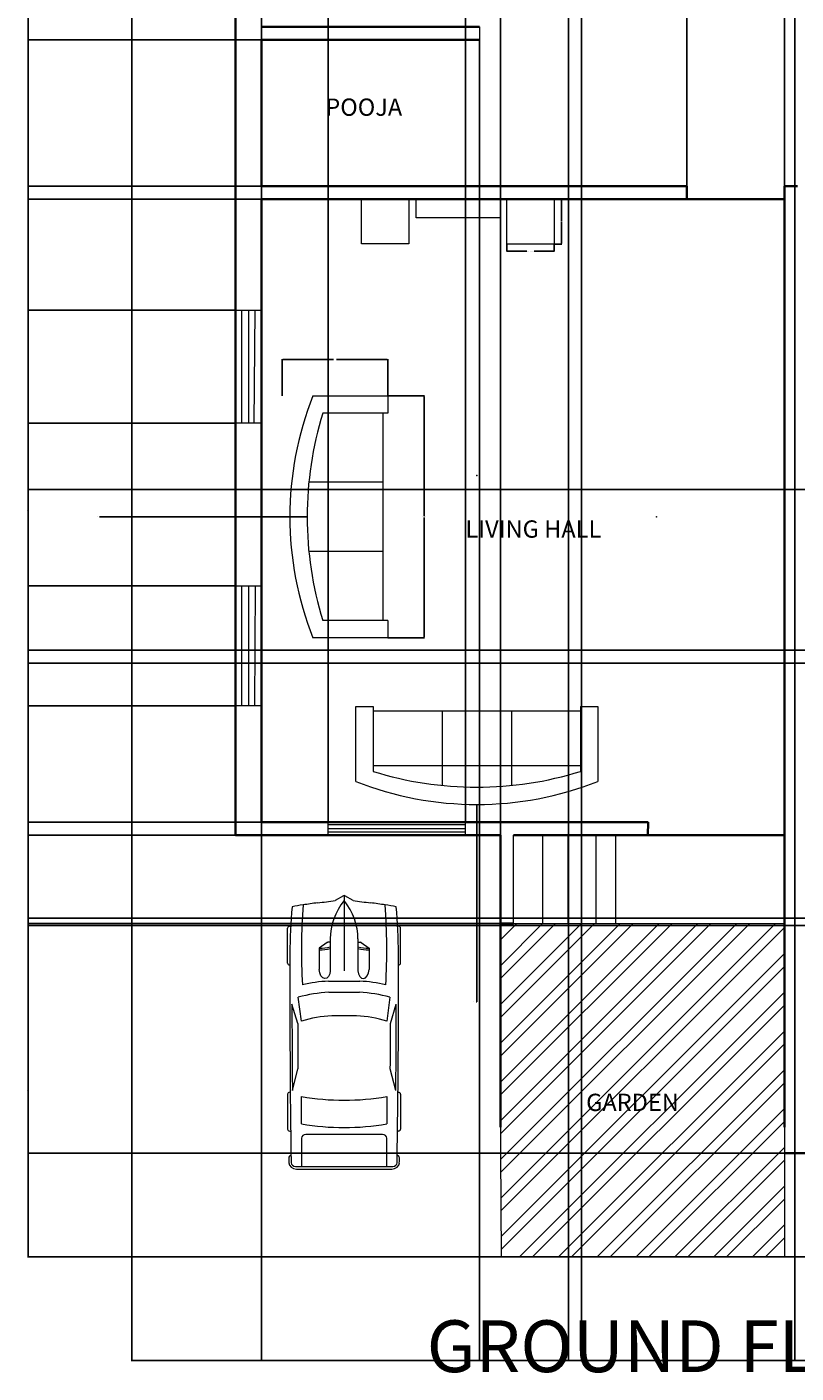
# Model space of a CAD drawing. Units: inches. Extents: x 2621 to 3621, y 1701 to 2465.
# Tile 1 of 6: x 2621 to 2888, y 1701 to 2169. Entities that reach past the tile are written whole.
import ezdxf

# ---------------------------------------------------------------- set-up
doc = ezdxf.new("R2010")
doc.units = ezdxf.units.IN
for name, color, linetype, lineweight in [('A-ANNO-DIMS', 2, 'Continuous', 18), ('A-ANNO-TEXT', 7, 'Continuous', 25), ('A-AREA-IDEN', 7, 'Continuous', 18), ('A-DOOR', 3, 'Continuous', 18), ('A-FLOR-STRS', 30, 'Continuous', 18), ('A-FURN', 8, 'Continuous', 18), ('A-GLAZ', 4, 'Continuous', 18), ('A-WALL', 7, 'Continuous', 35), ('C-PRKG-VEHI', 8, 'Continuous', 13), ('C-PROP', 8, 'Continuous', 25), ('L-PLNT', 94, 'Continuous', 18), ('L-PLNT-PATT', 9, 'Continuous', 13)]:
    doc.layers.add(name, color=color, linetype=linetype, lineweight=lineweight)
doc.styles.get("Standard").update_dxf_attribs({"font": 'arial.ttf'})
doc.dimstyles.get("Standard").update_dxf_attribs({"dimtxt": 0.18, "dimasz": 0.18, "dimexe": 0.18, "dimexo": 0.0625, "dimgap": 0.09, "dimtad": 0, "dimtih": 1, "dimtoh": 1, "dimdec": 4, "dimzin": 0, "dimdsep": 46, "dimtxsty": 'Standard', "dimcen": 0.09, "dimadec": 0, "dimazin": 0, "dimtfac": 1, "dimtdec": 4, "dimtofl": 0, "dimtmove": 0, "dimatfit": 3, "dimfxl": 1, "dimtolj": 1, "dimtzin": 0, "dimarcsym": 0})

# ---------------------------------------------------------------- blocks, each defined once
blk = doc.blocks.new('Sofa - Roundback 7 ft.')
for p, q in [((-12.00002, -32.4421), (-12.00003, -6.5971)), ((11.99997, -32.4421), (11.99998, -6.5971)), ((-36.000027, -34), (-36.000027, -11.4696)), ((-35.999844, -13.3819), (35.9998, -13.3819)), ((35.99998, -34), (35.99998, -11.4696)), ((-36.000027, -32.4421), (35.99998, -32.4421))]:
    blk.add_line(p, q)
for points in [[(-36.000027, -34), (-42.000027, -34), (-42.000027, -8)], [(41.99998, -8), (41.99998, -34), (35.99998, -34)]]:
    blk.add_lwpolyline(points)
for centre, radius, start, end in [((0, -114.25), 114.25, 68.43141, 111.5686), ((-0.00001, -127.1968), 121.1968, 72.72033, 107.2797)]:
    blk.add_arc(centre, radius, start, end)
blk = doc.blocks.new('*U5')
for p, q in [((21.1, 37.41), (21.1, 36.83)), ((46.55, 38.89), (22.35, 38.89)), ((47.8, 37.39), (47.8, 37.41)), ((135.45, 37.07), (135.45, 37.41)), ((136.7, 38.89), (160.9, 38.89)), ((162.15, 37.41), (162.15, 36.77)), ((70.03, 31.54), (86.41, 29.35)), ((87.99, 31.87), (74.76, 35.92)), ((134.31, 35.6), (119.29, 31.78)), ((138.42, 29.35), (157.25, 29.35)), ((186.47, 29.35), (167.01, 29.35)), ((186.47, -33.5), (186.47, 33.5)), ((188.4, -32.76), (188.4, 32.76)), ((164.52, 26.39), (164.52, -26.39)), ((29.77, 9.51), (51.68, 9.51)), ((32.12, 9.51), (32.12, 11.15)), ((32.27, 11.63), (36.13, 17.17)), ((36.13, 17.17), (50.94, 17.17)), ((58.92, -10.77), (58.92, 10.77)), ((66.55, -10.53), (66.55, 10.53)), ((186.47, -10.53), (186.47, 10.53)), ((3.27, 6.13), (0.1, 0.41)), ((82.74, 8.5), (82.74, -8.5)), ((0, 0), (51.68, 0)), ((0.1, -0.41), (3.27, -6.13)), ((29.77, -9.51), (51.68, -9.51)), ((32.12, -9.51), (32.12, -11.15)), ((32.27, -11.63), (36.13, -17.17)), ((36.13, -17.17), (50.94, -17.17)), ((21.1, -37.41), (21.1, -36.83)), ((86.41, -29.35), (70.03, -31.54)), ((87.99, -31.87), (74.76, -35.92)), ((134.31, -35.6), (119.29, -31.78)), ((135.45, -37.07), (135.45, -37.41)), ((157.25, -29.35), (138.42, -29.35)), ((162.15, -37.41), (162.15, -36.77)), ((167.01, -29.35), (186.47, -29.35)), ((46.55, -38.89), (22.35, -38.89)), ((47.8, -37.39), (47.8, -37.41)), ((136.7, -38.89), (160.9, -38.89))]:
    blk.add_line(p, q)
for centre, major_axis, ratio, start_param, end_param in [((41.19, -490.86), (0, 528.23), 0.842304, 0.00281, 0.075598), ((22.35, 37.41), (0, -1.48), 0.842304, 3.141593, 4.712389), ((64.48, -10555.62), (0, 10593.03), 0.842304, -0.013397, 0.002797), ((46.55, 37.41), (0, 1.48), 0.842304, -1.570796, 0), ((136.7, 37.41), (0, -1.48), 0.842304, 3.141593, 4.712389), ((160.9, 37.41), (0, 1.48), 0.842304, -1.570796, 0), ((180.63, 35.84), (0, 2.22), 0.842304, -0.013017, 1.249894), ((64.48, -10556.36), (0, 10595.31), 0.842304, -0.013397, -0.013017), ((183.98, 32.76), (0, -5.25), 0.842304, 1.570796, 3.128196), ((259.18, -27.52), (0, -305.3), 0.842304, 4.528606, 4.561838), ((266.03, -27.52), (0, 313.31), 0.842304, 1.367076, 1.39176), ((37.47, -593.96), (0, -623.33), 0.842304, 3.096046, 3.200911), ((134.4, 5.39), (0, -89.78), 0.842304, 4.449482, 4.652344), ((135.29, 5.39), (0, 81.77), 0.842304, 1.245306, 1.50788), ((64.48, -10555.62), (0, -10591.55), 0.842304, 3.133765, 3.140441), ((149.6, 2.8), (0, -79.58), 0.842304, 4.372215, 4.640744), ((95.79, -3666.35), (0, -3698.24), 0.842304, 3.134049, 3.144098), ((17.08, 0), (0, 147.02), 0.842304, 4.511394, 4.913384), ((35.91, 0), (0, 147.02), 0.842304, 4.511394, 4.913384), ((167.01, 26.39), (0, 2.96), 0.842304, 0, 1.570796), ((183.98, 33.5), (0, -2.96), 0.842304, 1.570796, 3.128196), ((-204.49, 52.4), (0, -250.96), 0.842304, 1.385369, 1.434372), ((29.77, -46.66), (0, 56.17), 0.842304, 0, 0.590319), ((32.75, 11.15), (0, 0.74), 0.842304, 0.879714, 1.570796), ((13.04, 17.01), (0, 27.42), 0.842304, 4.435146, 4.718221), ((14.2, 17.01), (0, 27.42), 0.842304, 4.435146, 4.718221), ((50.79, 13.34), (6.34, -0.36), 0.603834, -1.395552, 1.581315), ((0.62, 0), (0, -0.74), 0.842304, 4.131459, 5.293319), ((-204.49, -52.4), (0, 250.96), 0.842304, -1.434372, -1.385369), ((29.77, 46.66), (0, 56.17), 0.842304, 2.551274, 3.141593), ((149.6, -2.8), (0, -79.58), 0.842304, -1.499151, -1.230623), ((259.18, 27.52), (0, 305.3), 0.842304, 1.721348, 1.754579), ((32.75, -11.15), (0, -0.74), 0.842304, 4.712389, 5.403472), ((13.04, -17.01), (0, -27.42), 0.842304, 1.564964, 1.848039), ((14.2, -17.01), (0, -27.42), 0.842304, 1.564964, 1.848039), ((134.4, -5.39), (0, -89.78), 0.842304, -1.510751, -1.307889), ((135.29, -5.39), (0, -81.77), 0.842304, -1.50788, -1.245306), ((167.01, -26.39), (0, -2.96), 0.842304, 4.712389, 6.283185), ((266.03, 27.52), (0, 313.31), 0.842304, 1.749832, 1.774517), ((37.47, 593.96), (0, -623.33), 0.842304, -0.059319, 0.045547), ((41.19, 490.86), (0, -528.23), 0.842304, -0.075598, -0.00281), ((64.48, 10555.62), (0, 10593.03), 0.842304, 3.138796, 3.15499), ((64.48, 10555.62), (0, -10591.55), 0.842304, 0.001152, 0.007828), ((95.79, 3666.35), (0, -3698.24), 0.842304, -0.002505, 0.007544), ((180.63, -35.84), (0, -2.22), 0.842304, -1.249894, 0.013017), ((183.98, -33.5), (0, 2.96), 0.842304, 3.15499, 4.712389), ((183.98, -32.76), (0, -5.25), 0.842304, 0.013397, 1.570796), ((22.35, -37.41), (0, 1.48), 0.842304, 1.570796, 3.141593), ((46.55, -37.41), (0, -1.48), 0.842304, 0, 1.570796), ((136.7, -37.41), (0, -1.48), 0.842304, -1.570796, 0), ((160.9, -37.41), (0, 1.48), 0.842304, 3.141593, 4.712389), ((64.48, 10556.36), (0, 10595.31), 0.842304, 3.15461, 3.15499)]:
    blk.add_ellipse(centre, major_axis=major_axis, ratio=ratio, start_param=start_param, end_param=end_param)
at = {"extrusion": (0, 0, -1)}
blk.add_ellipse((50.79, -13.34), major_axis=(6.34, 0.36), ratio=0.603834, start_param=-1.395552, end_param=1.581315, dxfattribs=at)
blk = doc.blocks.new('LOT-33X57')
for p, q in [((0, 0), (0, 684)), ((396, 0), (0, 0))]:
    blk.add_line(p, q)
blk = doc.blocks.new('FURN-LIVING-SIDE-UNIT')
blk.add_lwpolyline([(0, 15.51), (16.46, 15.51), (16.46, 0), (0, 0)], close=True)
blk = doc.blocks.new('*D17')
at = {"layer": 'A-ANNO-DIMS', "color": 0, "lineweight": -2, "transparency": 16777216}
for p, q in [((2746.41, 2040.43), (2759.13, 2040.43)), ((2758.95, 2040.25), (2758.95, 1998.61)), ((2758.95, 1956.61), (2758.95, 1998.24)), ((2746.41, 1956.43), (2759.13, 1956.43))]:
    blk.add_line(p, q, dxfattribs=at)
at = {"layer": 'A-ANNO-DIMS', "color": 0, "transparency": 16777216}
for points in [[(2758.92, 2040.25), (2758.98, 2040.25), (2758.95, 2040.43)], [(2758.92, 1956.61), (2758.98, 1956.61), (2758.95, 1956.43)]]:
    blk.add_solid(points, dxfattribs=at)
at = {"layer": 'Defpoints', "color": 0, "transparency": 16777216}
for p in [(2746.35, 2040.43), (2758.95, 2040.43), (2746.35, 1956.43)]:
    blk.add_point(p, dxfattribs=at)
at = {"layer": 'A-ANNO-DIMS', "color": 0, "transparency": 16777216, "insert": (2758.95, 1998.43), "char_height": 0.18, "attachment_point": 5}
blk.add_mtext('\\A1;SOFA 84 TYP.', dxfattribs=at)
blk = doc.blocks.new('*D18')
at = {"layer": 'A-ANNO-DIMS', "color": 0, "lineweight": -2, "transparency": 16777216}
for p, q in [((2709.69, 2040.49), (2709.69, 2053.21)), ((2709.87, 2053.03), (2727.49, 2053.03)), ((2746.17, 2053.03), (2728.55, 2053.03)), ((2746.35, 2040.49), (2746.35, 2053.21))]:
    blk.add_line(p, q, dxfattribs=at)
at = {"layer": 'A-ANNO-DIMS', "color": 0, "transparency": 16777216}
for points in [[(2709.87, 2053.06), (2709.87, 2053), (2709.69, 2053.03)], [(2746.17, 2053.06), (2746.17, 2053), (2746.35, 2053.03)]]:
    blk.add_solid(points, dxfattribs=at)
at = {"layer": 'Defpoints', "color": 0, "transparency": 16777216}
for p in [(2709.69, 2053.03), (2709.69, 2040.43), (2746.35, 2040.43)]:
    blk.add_point(p, dxfattribs=at)
at = {"layer": 'A-ANNO-DIMS', "color": 0, "transparency": 16777216, "insert": (2728.02, 2053.03), "char_height": 0.18, "attachment_point": 5}
blk.add_mtext('\\A1;37 TYP.', dxfattribs=at)
blk = doc.blocks.new('*D31')
at = {"layer": 'A-ANNO-DIMS', "color": 0, "lineweight": -2, "transparency": 16777216}
for p, q in [((2787.64, 2093.1), (2787.64, 2090.52)), ((2787.82, 2090.7), (2794.59, 2090.7)), ((2803.93, 2090.7), (2797.16, 2090.7)), ((2804.11, 2093.1), (2804.11, 2090.52))]:
    blk.add_line(p, q, dxfattribs=at)
at = {"layer": 'A-ANNO-DIMS', "color": 0, "transparency": 16777216}
for points in [[(2787.82, 2090.73), (2787.82, 2090.67), (2787.64, 2090.7)], [(2803.93, 2090.73), (2803.93, 2090.67), (2804.11, 2090.7)]]:
    blk.add_solid(points, dxfattribs=at)
at = {"layer": 'Defpoints', "color": 0, "transparency": 16777216}
for p in [(2787.64, 2093.17), (2804.11, 2093.17), (2804.11, 2090.7)]:
    blk.add_point(p, dxfattribs=at)
at = {"layer": 'A-ANNO-DIMS', "color": 0, "transparency": 16777216, "insert": (2795.87, 2090.7), "char_height": 0.18, "attachment_point": 5}
blk.add_mtext('\\A1;SIDE TABLE 16 TYP.', dxfattribs=at)
blk = doc.blocks.new('*D32')
at = {"layer": 'A-ANNO-DIMS', "color": 0, "lineweight": -2, "transparency": 16777216}
for p, q in [((2804.17, 2108.67), (2806.76, 2108.67)), ((2806.58, 2108.49), (2806.58, 2101.1)), ((2806.58, 2093.35), (2806.58, 2100.74)), ((2804.17, 2093.17), (2806.76, 2093.17))]:
    blk.add_line(p, q, dxfattribs=at)
at = {"layer": 'A-ANNO-DIMS', "color": 0, "transparency": 16777216}
for points in [[(2806.55, 2108.49), (2806.61, 2108.49), (2806.58, 2108.67)], [(2806.55, 2093.35), (2806.61, 2093.35), (2806.58, 2093.17)]]:
    blk.add_solid(points, dxfattribs=at)
at = {"layer": 'Defpoints', "color": 0, "transparency": 16777216}
for p in [(2804.11, 2108.67), (2806.58, 2108.67), (2804.11, 2093.17)]:
    blk.add_point(p, dxfattribs=at)
at = {"layer": 'A-ANNO-DIMS', "color": 0, "transparency": 16777216, "insert": (2806.58, 2100.92), "char_height": 0.18, "attachment_point": 5}
blk.add_mtext('\\A1;16 TYP.', dxfattribs=at)
blk = doc.blocks.new('*D35')
at = {"layer": 'A-ANNO-DIMS', "color": 0, "lineweight": -2, "transparency": 16777216}
for p, q in [((2657.52, 1741.34), (2657.52, 1705.2)), ((3053.52, 1741.34), (3053.52, 1705.2)), ((2657.7, 1705.38), (2855.23, 1705.38)), ((3053.34, 1705.38), (2855.81, 1705.38))]:
    blk.add_line(p, q, dxfattribs=at)
at = {"layer": 'A-ANNO-DIMS', "color": 0, "transparency": 16777216}
for points in [[(2657.7, 1705.41), (2657.7, 1705.35), (2657.52, 1705.38)], [(3053.34, 1705.41), (3053.34, 1705.35), (3053.52, 1705.38)]]:
    blk.add_solid(points, dxfattribs=at)
at = {"layer": 'Defpoints', "color": 0, "transparency": 16777216}
for p in [(2657.52, 1741.4), (3053.52, 1741.4), (3053.52, 1705.38)]:
    blk.add_point(p, dxfattribs=at)
at = {"layer": 'A-ANNO-DIMS', "color": 0, "transparency": 16777216, "insert": (2855.52, 1705.38), "char_height": 0.18, "attachment_point": 5}
blk.add_mtext('\\A1;396', dxfattribs=at)
blk = doc.blocks.new('*D36')
at = {"layer": 'A-ANNO-DIMS', "color": 0, "lineweight": -2, "transparency": 16777216}
for p, q in [((2657.46, 2425.4), (2621.31, 2425.4)), ((2621.49, 2425.22), (2621.49, 2083.58)), ((2621.49, 1741.58), (2621.49, 2083.22)), ((2657.46, 1741.4), (2621.31, 1741.4))]:
    blk.add_line(p, q, dxfattribs=at)
at = {"layer": 'A-ANNO-DIMS', "color": 0, "transparency": 16777216}
for points in [[(2621.46, 2425.22), (2621.52, 2425.22), (2621.49, 2425.4)], [(2621.46, 1741.58), (2621.52, 1741.58), (2621.49, 1741.4)]]:
    blk.add_solid(points, dxfattribs=at)
at = {"layer": 'Defpoints', "color": 0, "transparency": 16777216}
for p in [(2621.49, 2425.4), (2657.52, 2425.4), (2657.52, 1741.4)]:
    blk.add_point(p, dxfattribs=at)
at = {"layer": 'A-ANNO-DIMS', "color": 0, "transparency": 16777216, "insert": (2621.49, 2083.4), "char_height": 0.18, "attachment_point": 5}
blk.add_mtext('\\A1;684', dxfattribs=at)
blk = doc.blocks.new('*D42')
at = {"layer": 'A-ANNO-DIMS', "color": 0, "lineweight": -2, "transparency": 16777216}
for p, q in [((2702.52, 2380.34), (2702.52, 1705.2)), ((2809.02, 2380.34), (2809.02, 1705.2)), ((2702.7, 1705.38), (2755.38, 1705.38)), ((2808.84, 1705.38), (2756.15, 1705.38))]:
    blk.add_line(p, q, dxfattribs=at)
at = {"layer": 'A-ANNO-DIMS', "color": 0, "transparency": 16777216}
for points in [[(2702.7, 1705.41), (2702.7, 1705.35), (2702.52, 1705.38)], [(2808.84, 1705.41), (2808.84, 1705.35), (2809.02, 1705.38)]]:
    blk.add_solid(points, dxfattribs=at)
at = {"layer": 'Defpoints', "color": 0, "transparency": 16777216}
for p in [(2702.52, 2380.4), (2809.02, 2380.4), (2809.02, 1705.38)]:
    blk.add_point(p, dxfattribs=at)
at = {"layer": 'A-ANNO-DIMS', "color": 0, "transparency": 16777216, "insert": (2755.77, 1705.38), "char_height": 0.18, "attachment_point": 5}
blk.add_mtext('\\A1;106.5', dxfattribs=at)
blk = doc.blocks.new('*D43')
at = {"layer": 'A-ANNO-DIMS', "color": 0, "lineweight": -2, "transparency": 16777216}
for p, q in [((2813.52, 2380.34), (2813.52, 1705.2)), ((2887.57, 2380.34), (2887.57, 1705.2)), ((2813.7, 1705.38), (2850.15, 1705.38)), ((2887.39, 1705.38), (2850.94, 1705.38))]:
    blk.add_line(p, q, dxfattribs=at)
at = {"layer": 'A-ANNO-DIMS', "color": 0, "transparency": 16777216}
for points in [[(2813.7, 1705.41), (2813.7, 1705.35), (2813.52, 1705.38)], [(2887.39, 1705.41), (2887.39, 1705.35), (2887.57, 1705.38)]]:
    blk.add_solid(points, dxfattribs=at)
at = {"layer": 'Defpoints', "color": 0, "transparency": 16777216}
for p in [(2813.52, 2380.4), (2887.57, 2380.4), (2887.57, 1705.38)]:
    blk.add_point(p, dxfattribs=at)
at = {"layer": 'A-ANNO-DIMS', "color": 0, "transparency": 16777216, "insert": (2850.55, 1705.38), "char_height": 0.18, "attachment_point": 5}
blk.add_mtext('\\A1;74.05', dxfattribs=at)
blk = doc.blocks.new('*D49')
at = {"layer": 'A-ANNO-DIMS', "color": 0, "lineweight": -2, "transparency": 16777216}
for p, q in [((2702.52, 2164.01), (2702.52, 1705.2)), ((2778.15, 2164.01), (2778.15, 1705.2)), ((2702.7, 1705.38), (2739.94, 1705.38)), ((2777.97, 1705.38), (2740.73, 1705.38))]:
    blk.add_line(p, q, dxfattribs=at)
at = {"layer": 'A-ANNO-DIMS', "color": 0, "transparency": 16777216}
for points in [[(2702.7, 1705.41), (2702.7, 1705.35), (2702.52, 1705.38)], [(2777.97, 1705.41), (2777.97, 1705.35), (2778.15, 1705.38)]]:
    blk.add_solid(points, dxfattribs=at)
at = {"layer": 'Defpoints', "color": 0, "transparency": 16777216}
for p in [(2702.52, 2164.07), (2778.15, 2164.07), (2778.15, 1705.38)]:
    blk.add_point(p, dxfattribs=at)
at = {"layer": 'A-ANNO-DIMS', "color": 0, "transparency": 16777216, "insert": (2740.33, 1705.38), "char_height": 0.18, "attachment_point": 5}
blk.add_mtext('\\A1;75.63', dxfattribs=at)
blk = doc.blocks.new('*D50')
at = {"layer": 'A-ANNO-DIMS', "color": 0, "lineweight": -2, "transparency": 16777216}
for p, q in [((2702.46, 2164.07), (2621.31, 2164.07)), ((2621.49, 2163.89), (2621.49, 2138.84)), ((2621.49, 2113.43), (2621.49, 2138.48)), ((2702.46, 2113.25), (2621.31, 2113.25))]:
    blk.add_line(p, q, dxfattribs=at)
at = {"layer": 'A-ANNO-DIMS', "color": 0, "transparency": 16777216}
for points in [[(2621.46, 2163.89), (2621.52, 2163.89), (2621.49, 2164.07)], [(2621.46, 2113.43), (2621.52, 2113.43), (2621.49, 2113.25)]]:
    blk.add_solid(points, dxfattribs=at)
at = {"layer": 'Defpoints', "color": 0, "transparency": 16777216}
for p in [(2621.49, 2164.07), (2702.52, 2164.07), (2702.52, 2113.25)]:
    blk.add_point(p, dxfattribs=at)
at = {"layer": 'A-ANNO-DIMS', "color": 0, "transparency": 16777216, "insert": (2621.49, 2138.66), "char_height": 0.18, "attachment_point": 5}
blk.add_mtext('\\A1;50.82', dxfattribs=at)
blk = doc.blocks.new('*D51')
at = {"layer": 'A-ANNO-DIMS', "color": 0, "lineweight": -2, "transparency": 16777216}
for p, q in [((2702.46, 2108.75), (2621.31, 2108.75)), ((2621.49, 2108.57), (2621.49, 2000.76)), ((2621.49, 1892.58), (2621.49, 2000.39)), ((2702.46, 1892.4), (2621.31, 1892.4))]:
    blk.add_line(p, q, dxfattribs=at)
at = {"layer": 'A-ANNO-DIMS', "color": 0, "transparency": 16777216}
for points in [[(2621.46, 2108.57), (2621.52, 2108.57), (2621.49, 2108.75)], [(2621.46, 1892.58), (2621.52, 1892.58), (2621.49, 1892.4)]]:
    blk.add_solid(points, dxfattribs=at)
at = {"layer": 'Defpoints', "color": 0, "transparency": 16777216}
for p in [(2621.49, 2108.75), (2702.52, 2108.75), (2702.52, 1892.4)]:
    blk.add_point(p, dxfattribs=at)
at = {"layer": 'A-ANNO-DIMS', "color": 0, "transparency": 16777216, "insert": (2621.49, 2000.58), "char_height": 0.18, "attachment_point": 5}
blk.add_mtext('\\A1;216.35', dxfattribs=at)
blk = doc.blocks.new('*D52')
at = {"layer": 'A-ANNO-DIMS', "color": 0, "lineweight": -2, "transparency": 16777216}
for p, q in [((2702.52, 1892.46), (2702.52, 2461.61)), ((2702.7, 2461.43), (2792.8, 2461.43)), ((2883.82, 2461.43), (2793.71, 2461.43)), ((2884, 1887.96), (2884, 2461.61))]:
    blk.add_line(p, q, dxfattribs=at)
at = {"layer": 'A-ANNO-DIMS', "color": 0, "transparency": 16777216}
for points in [[(2702.7, 2461.46), (2702.7, 2461.4), (2702.52, 2461.43)], [(2883.82, 2461.46), (2883.82, 2461.4), (2884, 2461.43)]]:
    blk.add_solid(points, dxfattribs=at)
at = {"layer": 'Defpoints', "color": 0, "transparency": 16777216}
for p in [(2884, 2461.43), (2702.52, 1892.4), (2884, 1887.9)]:
    blk.add_point(p, dxfattribs=at)
at = {"layer": 'A-ANNO-DIMS', "color": 0, "transparency": 16777216, "insert": (2793.26, 2461.43), "char_height": 0.18, "attachment_point": 5}
blk.add_mtext('\\A1;181.48', dxfattribs=at)
blk = doc.blocks.new('*D54')
at = {"layer": 'A-ANNO-DIMS', "color": 0, "lineweight": -2, "transparency": 16777216}
for p, q in [((3008.46, 1856.54), (2621.31, 1856.54)), ((2621.49, 1856.36), (2621.49, 1817.15)), ((2621.49, 1777.58), (2621.49, 1816.79)), ((3008.46, 1777.4), (2621.31, 1777.4))]:
    blk.add_line(p, q, dxfattribs=at)
at = {"layer": 'A-ANNO-DIMS', "color": 0, "transparency": 16777216}
for points in [[(2621.46, 1856.36), (2621.52, 1856.36), (2621.49, 1856.54)], [(2621.46, 1777.58), (2621.52, 1777.58), (2621.49, 1777.4)]]:
    blk.add_solid(points, dxfattribs=at)
at = {"layer": 'Defpoints', "color": 0, "transparency": 16777216}
for p in [(2621.49, 1856.54), (3008.52, 1856.54), (3008.52, 1777.4)]:
    blk.add_point(p, dxfattribs=at)
at = {"layer": 'A-ANNO-DIMS', "color": 0, "transparency": 16777216, "insert": (2621.49, 1816.97), "char_height": 0.18, "attachment_point": 5}
blk.add_mtext('\\A1;79.14', dxfattribs=at)
blk = doc.blocks.new('*D55')
at = {"layer": 'A-ANNO-DIMS', "color": 0, "lineweight": -2, "transparency": 16777216}
for p, q in [((3008.46, 1947.58), (2621.31, 1947.58)), ((2621.49, 1947.4), (2621.49, 1903.51)), ((2621.49, 1859.26), (2621.49, 1903.15)), ((3008.46, 1859.08), (2621.31, 1859.08))]:
    blk.add_line(p, q, dxfattribs=at)
at = {"layer": 'A-ANNO-DIMS', "color": 0, "transparency": 16777216}
for points in [[(2621.46, 1947.4), (2621.52, 1947.4), (2621.49, 1947.58)], [(2621.46, 1859.26), (2621.52, 1859.26), (2621.49, 1859.08)]]:
    blk.add_solid(points, dxfattribs=at)
at = {"layer": 'Defpoints', "color": 0, "transparency": 16777216}
for p in [(2621.49, 1947.58), (3008.52, 1947.58), (3008.52, 1859.08)]:
    blk.add_point(p, dxfattribs=at)
at = {"layer": 'A-ANNO-DIMS', "color": 0, "transparency": 16777216, "insert": (2621.49, 1903.33), "char_height": 0.18, "attachment_point": 5}
blk.add_mtext('\\A1;88.5', dxfattribs=at)
blk = doc.blocks.new('*D58')
at = {"layer": 'A-ANNO-DIMS', "color": 0, "lineweight": -2, "transparency": 16777216}
for p, q in [((2933.41, 2007.9), (2621.31, 2007.9)), ((2621.49, 2007.72), (2621.49, 1980.17)), ((2621.49, 1952.26), (2621.49, 1979.81)), ((2933.41, 1952.08), (2621.31, 1952.08))]:
    blk.add_line(p, q, dxfattribs=at)
at = {"layer": 'A-ANNO-DIMS', "color": 0, "transparency": 16777216}
for points in [[(2621.46, 2007.72), (2621.52, 2007.72), (2621.49, 2007.9)], [(2621.46, 1952.26), (2621.52, 1952.26), (2621.49, 1952.08)]]:
    blk.add_solid(points, dxfattribs=at)
at = {"layer": 'Defpoints', "color": 0, "transparency": 16777216}
for p in [(2621.49, 2007.9), (2933.47, 2007.9), (2933.47, 1952.08)]:
    blk.add_point(p, dxfattribs=at)
at = {"layer": 'A-ANNO-DIMS', "color": 0, "transparency": 16777216, "insert": (2621.49, 1979.99), "char_height": 0.18, "attachment_point": 5}
blk.add_mtext('\\A1;55.82', dxfattribs=at)
blk = doc.blocks.new('*D61')
at = {"layer": 'A-ANNO-DIMS', "color": 0, "lineweight": -2, "transparency": 16777216}
for p, q in [((2785.46, 1857.23), (2785.46, 2461.61)), ((2785.64, 2461.43), (2834.33, 2461.43)), ((2883.82, 2461.43), (2835.12, 2461.43)), ((2884, 1857.23), (2884, 2461.61))]:
    blk.add_line(p, q, dxfattribs=at)
at = {"layer": 'A-ANNO-DIMS', "color": 0, "transparency": 16777216}
for points in [[(2785.64, 2461.46), (2785.64, 2461.4), (2785.46, 2461.43)], [(2883.82, 2461.46), (2883.82, 2461.4), (2884, 2461.43)]]:
    blk.add_solid(points, dxfattribs=at)
at = {"layer": 'Defpoints', "color": 0, "transparency": 16777216}
for p in [(2884, 2461.43), (2785.46, 1857.17), (2884, 1857.17)]:
    blk.add_point(p, dxfattribs=at)
at = {"layer": 'A-ANNO-DIMS', "color": 0, "transparency": 16777216, "insert": (2834.73, 2461.43), "char_height": 0.18, "attachment_point": 5}
blk.add_mtext('\\A1;98.54', dxfattribs=at)
blk = doc.blocks.new('*D62')
at = {"layer": 'A-ANNO-DIMS', "color": 0, "lineweight": -2, "transparency": 16777216}
for p, q in [((2785.4, 1857.17), (2621.31, 1857.17)), ((2621.49, 1856.99), (2621.49, 1799.47)), ((2621.49, 1741.58), (2621.49, 1799.1)), ((2785.66, 1741.4), (2621.31, 1741.4))]:
    blk.add_line(p, q, dxfattribs=at)
at = {"layer": 'A-ANNO-DIMS', "color": 0, "transparency": 16777216}
for points in [[(2621.46, 1856.99), (2621.52, 1856.99), (2621.49, 1857.17)], [(2621.46, 1741.58), (2621.52, 1741.58), (2621.49, 1741.4)]]:
    blk.add_solid(points, dxfattribs=at)
at = {"layer": 'Defpoints', "color": 0, "transparency": 16777216}
for p in [(2621.49, 1857.17), (2785.46, 1857.17), (2785.72, 1741.4)]:
    blk.add_point(p, dxfattribs=at)
at = {"layer": 'A-ANNO-DIMS', "color": 0, "transparency": 16777216, "insert": (2621.49, 1799.28), "char_height": 0.18, "attachment_point": 5}
blk.add_mtext('\\A1;115.77', dxfattribs=at)
blk = doc.blocks.new('*D87')
at = {"layer": 'A-ANNO-DIMS', "color": 0, "lineweight": -2, "transparency": 16777216}
for p, q in [((2693.46, 1932.75), (2621.31, 1932.75)), ((2621.49, 1932.57), (2621.49, 1910.51)), ((2621.49, 1888.08), (2621.49, 1910.14)), ((2693.46, 1887.9), (2621.31, 1887.9))]:
    blk.add_line(p, q, dxfattribs=at)
at = {"layer": 'A-ANNO-DIMS', "color": 0, "transparency": 16777216}
for points in [[(2621.46, 1932.57), (2621.52, 1932.57), (2621.49, 1932.75)], [(2621.46, 1888.08), (2621.52, 1888.08), (2621.49, 1887.9)]]:
    blk.add_solid(points, dxfattribs=at)
at = {"layer": 'Defpoints', "color": 0, "transparency": 16777216}
for p in [(2621.49, 1932.75), (2693.52, 1932.75), (2693.52, 1887.9)]:
    blk.add_point(p, dxfattribs=at)
at = {"layer": 'A-ANNO-DIMS', "color": 0, "transparency": 16777216, "insert": (2621.49, 1910.32), "char_height": 0.18, "attachment_point": 5}
blk.add_mtext('\\A1;44.85', dxfattribs=at)
blk = doc.blocks.new('*D88')
at = {"layer": 'A-ANNO-DIMS', "color": 0, "lineweight": -2, "transparency": 16777216}
for p, q in [((2693.46, 1974.42), (2621.31, 1974.42)), ((2621.49, 1974.24), (2621.49, 1953.77)), ((2621.49, 1932.93), (2621.49, 1953.4)), ((2693.46, 1932.75), (2621.31, 1932.75))]:
    blk.add_line(p, q, dxfattribs=at)
at = {"layer": 'A-ANNO-DIMS', "color": 0, "transparency": 16777216}
for points in [[(2621.46, 1974.24), (2621.52, 1974.24), (2621.49, 1974.42)], [(2621.46, 1932.93), (2621.52, 1932.93), (2621.49, 1932.75)]]:
    blk.add_solid(points, dxfattribs=at)
at = {"layer": 'Defpoints', "color": 0, "transparency": 16777216}
for p in [(2621.49, 1974.42), (2693.52, 1974.42), (2693.52, 1932.75)]:
    blk.add_point(p, dxfattribs=at)
at = {"layer": 'A-ANNO-DIMS', "color": 0, "transparency": 16777216, "insert": (2621.49, 1953.59), "char_height": 0.18, "attachment_point": 5}
blk.add_mtext('\\A1;41.67', dxfattribs=at)
blk = doc.blocks.new('*D89')
at = {"layer": 'A-ANNO-DIMS', "color": 0, "lineweight": -2, "transparency": 16777216}
for p, q in [((2693.46, 2030.98), (2621.31, 2030.98)), ((2621.49, 2030.8), (2621.49, 2002.88)), ((2621.49, 1974.6), (2621.49, 2002.52)), ((2693.46, 1974.42), (2621.31, 1974.42))]:
    blk.add_line(p, q, dxfattribs=at)
at = {"layer": 'A-ANNO-DIMS', "color": 0, "transparency": 16777216}
for points in [[(2621.46, 2030.8), (2621.52, 2030.8), (2621.49, 2030.98)], [(2621.46, 1974.6), (2621.52, 1974.6), (2621.49, 1974.42)]]:
    blk.add_solid(points, dxfattribs=at)
at = {"layer": 'Defpoints', "color": 0, "transparency": 16777216}
for p in [(2621.49, 2030.98), (2693.52, 2030.98), (2693.52, 1974.42)]:
    blk.add_point(p, dxfattribs=at)
at = {"layer": 'A-ANNO-DIMS', "color": 0, "transparency": 16777216, "insert": (2621.49, 2002.7), "char_height": 0.18, "attachment_point": 5}
blk.add_mtext('\\A1;56.55', dxfattribs=at)
blk = doc.blocks.new('*D90')
at = {"layer": 'A-ANNO-DIMS', "color": 0, "lineweight": -2, "transparency": 16777216}
for p, q in [((2693.46, 2070.17), (2621.31, 2070.17)), ((2621.49, 2069.99), (2621.49, 2050.75)), ((2621.49, 2031.16), (2621.49, 2050.39)), ((2693.46, 2030.98), (2621.31, 2030.98))]:
    blk.add_line(p, q, dxfattribs=at)
at = {"layer": 'A-ANNO-DIMS', "color": 0, "transparency": 16777216}
for points in [[(2621.46, 2069.99), (2621.52, 2069.99), (2621.49, 2070.17)], [(2621.46, 2031.16), (2621.52, 2031.16), (2621.49, 2030.98)]]:
    blk.add_solid(points, dxfattribs=at)
at = {"layer": 'Defpoints', "color": 0, "transparency": 16777216}
for p in [(2621.49, 2070.17), (2693.52, 2070.17), (2693.52, 2030.98)]:
    blk.add_point(p, dxfattribs=at)
at = {"layer": 'A-ANNO-DIMS', "color": 0, "transparency": 16777216, "insert": (2621.49, 2050.57), "char_height": 0.18, "attachment_point": 5}
blk.add_mtext('\\A1;39.19', dxfattribs=at)
blk = doc.blocks.new('*D98')
at = {"layer": 'A-ANNO-DIMS', "color": 0, "lineweight": -2, "transparency": 16777216}
for p, q in [((2702.52, 1892.46), (2702.52, 2461.61)), ((2702.7, 2461.43), (2713.72, 2461.43)), ((2725.53, 2461.43), (2714.51, 2461.43)), ((2725.71, 1892.46), (2725.71, 2461.61))]:
    blk.add_line(p, q, dxfattribs=at)
at = {"layer": 'A-ANNO-DIMS', "color": 0, "transparency": 16777216}
for points in [[(2702.7, 2461.46), (2702.7, 2461.4), (2702.52, 2461.43)], [(2725.53, 2461.46), (2725.53, 2461.4), (2725.71, 2461.43)]]:
    blk.add_solid(points, dxfattribs=at)
at = {"layer": 'Defpoints', "color": 0, "transparency": 16777216}
for p in [(2725.71, 2461.43), (2702.52, 1892.4), (2725.71, 1892.4)]:
    blk.add_point(p, dxfattribs=at)
at = {"layer": 'A-ANNO-DIMS', "color": 0, "transparency": 16777216, "insert": (2714.11, 2461.43), "char_height": 0.18, "attachment_point": 5}
blk.add_mtext('\\A1;23.19', dxfattribs=at)
blk = doc.blocks.new('*D99')
at = {"layer": 'A-ANNO-DIMS', "color": 0, "lineweight": -2, "transparency": 16777216}
for p, q in [((2725.71, 1892.46), (2725.71, 2461.61)), ((2725.89, 2461.43), (2749.13, 2461.43)), ((2773.18, 2461.43), (2749.93, 2461.43)), ((2773.36, 1892.46), (2773.36, 2461.61))]:
    blk.add_line(p, q, dxfattribs=at)
at = {"layer": 'A-ANNO-DIMS', "color": 0, "transparency": 16777216}
for points in [[(2725.89, 2461.46), (2725.89, 2461.4), (2725.71, 2461.43)], [(2773.18, 2461.46), (2773.18, 2461.4), (2773.36, 2461.43)]]:
    blk.add_solid(points, dxfattribs=at)
at = {"layer": 'Defpoints', "color": 0, "transparency": 16777216}
for p in [(2773.36, 2461.43), (2725.71, 1892.4), (2773.36, 1892.4)]:
    blk.add_point(p, dxfattribs=at)
at = {"layer": 'A-ANNO-DIMS', "color": 0, "transparency": 16777216, "insert": (2749.53, 2461.43), "char_height": 0.18, "attachment_point": 5}
blk.add_mtext('\\A1;47.65', dxfattribs=at)
blk = doc.blocks.new('*D100')
at = {"layer": 'A-ANNO-DIMS', "color": 0, "lineweight": -2, "transparency": 16777216}
for p, q in [((2850.13, 2113.32), (2850.13, 2461.61)), ((2850.31, 2461.43), (2866.67, 2461.43)), ((2883.82, 2461.43), (2867.45, 2461.43)), ((2884, 2113.32), (2884, 2461.61))]:
    blk.add_line(p, q, dxfattribs=at)
at = {"layer": 'A-ANNO-DIMS', "color": 0, "transparency": 16777216}
for points in [[(2850.31, 2461.46), (2850.31, 2461.4), (2850.13, 2461.43)], [(2883.82, 2461.46), (2883.82, 2461.4), (2884, 2461.43)]]:
    blk.add_solid(points, dxfattribs=at)
at = {"layer": 'Defpoints', "color": 0, "transparency": 16777216}
for p in [(2884, 2461.43), (2850.13, 2113.25), (2884, 2113.25)]:
    blk.add_point(p, dxfattribs=at)
at = {"layer": 'A-ANNO-DIMS', "color": 0, "transparency": 16777216, "insert": (2867.06, 2461.43), "char_height": 0.18, "attachment_point": 5}
blk.add_mtext('\\A1;33.87', dxfattribs=at)
blk = doc.blocks.new('*D106')
at = {"layer": 'A-ANNO-DIMS', "color": 0, "lineweight": -2, "transparency": 16777216}
for p, q in [((2646.31, 1998.43), (2718.17, 1998.43)), ((2839.46, 1998.43), (2839.64, 1998.43)), ((2839.55, 1998.34), (2839.55, 1998.52))]:
    blk.add_line(p, q, dxfattribs=at)
at = {"layer": 'A-ANNO-DIMS', "color": 0, "transparency": 16777216}
blk.add_solid([(2718.17, 1998.46), (2718.17, 1998.4), (2718.35, 1998.43)], dxfattribs=at)
at = {"layer": 'Defpoints', "color": 0, "transparency": 16777216}
for p in [(2718.35, 1998.43), (2839.55, 1998.43)]:
    blk.add_point(p, dxfattribs=at)
at = {"layer": 'A-ANNO-DIMS', "color": 0, "transparency": 16777216, "insert": (2645.63, 1998.43), "char_height": 0.18, "attachment_point": 5}
blk.add_mtext('\\A1;2X R121.2', dxfattribs=at)
blk = doc.blocks.new('*D107')
at = {"layer": 'A-ANNO-DIMS', "color": 0, "lineweight": -2, "transparency": 16777216}
for p, q in [((2777.14, 2012.78), (2777.32, 2012.78)), ((2777.23, 2012.69), (2777.23, 2012.87)), ((2777.23, 1829.98), (2777.23, 1898.35)), ((2777.05, 1829.98), (2777.23, 1829.98))]:
    blk.add_line(p, q, dxfattribs=at)
at = {"layer": 'A-ANNO-DIMS', "color": 0, "transparency": 16777216}
blk.add_solid([(2777.2, 1898.35), (2777.26, 1898.35), (2777.23, 1898.53)], dxfattribs=at)
at = {"layer": 'Defpoints', "color": 0, "transparency": 16777216}
for p in [(2777.23, 2012.78), (2777.23, 1898.53)]:
    blk.add_point(p, dxfattribs=at)
at = {"layer": 'A-ANNO-DIMS', "color": 0, "transparency": 16777216, "insert": (2776.3, 1829.98), "char_height": 0.18, "attachment_point": 5}
blk.add_mtext('\\A1;2X R114.25', dxfattribs=at)

msp = doc.modelspace()

# ---------------------------------------------------------------- hatches: boundary and pattern name
at = {"layer": 'L-PLNT-PATT'}
h = msp.add_hatch(dxfattribs=at)
h.set_pattern_fill('ANSI32', color=256)
h.paths.add_polyline_path([(2883.995, 1857.1678), (2789.9592, 1857.1678), (2785.4592, 1857.1678), (2785.4592, 1786.4015), (2785.4592, 1777.4015), (2785.7201, 1741.4015), (2883.995, 1741.4015), (2883.995, 1786.4015)])

# ---------------------------------------------------------------- linework, layer by layer
at = {"layer": 'A-DOOR'}
msp.add_line((2778.1477, 2168.5709), (2778.1477, 2113.2527), dxfattribs=at)
at = {"layer": 'A-FLOR-STRS'}
for p, q in [((2789.9592, 1857.1678), (2789.9592, 1887.8987)), ((2800.1093, 1857.1678), (2800.1093, 1887.8987)), ((2808.9654, 1857.1678), (2808.9654, 1887.8987)), ((2818.6518, 1857.1678), (2818.6518, 1887.8987)), ((2825.466, 1857.1678), (2825.466, 1887.8987)), ((2789.9592, 1857.1678), (2883.995, 1857.1678))]:
    msp.add_line(p, q, dxfattribs=at)
at = {"layer": 'A-FURN'}
msp.add_lwpolyline([(2756.1697, 2108.7527), (2785.4943, 2108.7527), (2785.4943, 2102.2982), (2756.1697, 2102.2982)], close=True, dxfattribs=at)
at = {"layer": 'A-GLAZ'}
for p, q in [((2695.6642, 2030.9765), (2695.6642, 2070.168)), ((2698.0184, 2070.168), (2698.0184, 2030.9765)), ((2700.1954, 2070.168), (2699.828, 2030.9765)), ((2695.662, 1932.7498), (2695.7383, 1974.4218)), ((2698.0184, 1974.4218), (2698.0184, 1932.7498)), ((2700.2073, 1932.7498), (2700.3939, 1974.4218)), ((2725.7097, 1887.8987), (2725.7097, 1892.3987)), ((2773.3373, 1891.4514), (2725.7097, 1891.4514)), ((2725.7097, 1890.1487), (2773.312, 1890.1487)), ((2725.7097, 1889.0239), (2773.2901, 1889.0239)), ((2773.2683, 1887.8987), (2773.3557, 1892.3987))]:
    msp.add_line(p, q, dxfattribs=at)
for points in [[(2693.5184, 2070.168), (2702.5184, 2070.168), (2702.5184, 2030.9765), (2693.5184, 2030.9765)], [(2693.5184, 1974.4218), (2702.5184, 1974.4218), (2702.5184, 1932.7498), (2693.5184, 1932.7498)]]:
    msp.add_lwpolyline(points, close=True, dxfattribs=at)
at = {"layer": 'A-WALL'}
for p, q in [((2693.5184, 2425.4015), (2693.5184, 1887.8987)), ((2702.5184, 2168.5709), (2778.1477, 2168.5709)), ((2702.5184, 2164.0709), (2773.6477, 2164.0709)), ((2702.5184, 2164.0709), (2702.5184, 2113.2527)), ((2773.6477, 2164.0709), (2778.1477, 2164.0709)), ((2773.6477, 2113.2527), (2702.5184, 2113.2527)), ((2883.995, 2108.7527), (2702.5184, 2108.7527)), ((2702.5184, 2108.7527), (2702.5184, 1892.3987)), ((2773.6477, 2113.2527), (2778.1477, 2113.2527)), ((2850.1273, 2113.2527), (2778.1477, 2113.2527)), ((2850.1273, 2108.7527), (2850.1273, 2113.2527)), ((2883.995, 2012.3975), (2883.995, 2113.2527)), ((2883.995, 2113.2527), (2888.495, 2113.2527)), ((2883.995, 2012.3975), (2883.995, 1892.3987)), ((2789.9592, 1892.3987), (2702.5184, 1892.3987)), ((2836.6895, 1892.3987), (2789.9592, 1892.3987)), ((2836.5841, 1887.8987), (2836.6895, 1892.3987)), ((2883.995, 1892.3987), (2883.995, 1786.4015)), ((2702.5184, 1887.8987), (2693.5184, 1887.8987)), ((2785.4592, 1887.8987), (2702.5184, 1887.8987)), ((2785.4592, 1786.4015), (2785.4592, 1887.8987)), ((2883.209, 1887.8987), (2789.9592, 1887.8987)), ((2883.209, 1887.8987), (2883.995, 1887.8987)), ((2789.9592, 1857.1678), (2785.4592, 1857.1678)), ((3017.5184, 1777.4015), (2883.995, 1777.4015))]:
    msp.add_line(p, q, dxfattribs=at)
at = {"layer": 'L-PLNT'}
for p, q in [((2785.4592, 1786.4015), (2785.4592, 1777.4015)), ((2883.995, 1786.4015), (2883.995, 1741.4015)), ((2785.4592, 1777.4015), (2785.7201, 1741.4015))]:
    msp.add_line(p, q, dxfattribs=at)

# ---------------------------------------------------------------- block references
at = {"layer": 'A-FURN'}
for p in [(2737.248, 2093.246), (2787.6424, 2093.165)]:
    msp.add_blockref('FURN-LIVING-SIDE-UNIT', p, dxfattribs=at)
for p, rotation in [((2712.352, 1998.426), 90), ((2777.229, 1898.5258), 180)]:
    msp.add_blockref('Sofa - Roundback 7 ft.', p, dxfattribs=dict(at, rotation=rotation))
at = {"layer": 'C-PRKG-VEHI', "xscale": 0.5041519641766145, "yscale": 0.5041519641766145, "zscale": 0.5041519641766145, "rotation": 270}
msp.add_blockref('*U5', (2731.1959, 1866.8463), dxfattribs=at)
at = {"layer": 'C-PROP'}
msp.add_blockref('LOT-33X57', (2657.518, 1741.402), dxfattribs=at)

# ---------------------------------------------------------------- texts
at = {"layer": 'A-ANNO-TEXT', "insert": (2759.8469, 1719.3538), "char_height": 18, "attachment_point": 1}
msp.add_mtext_dynamic_manual_height_columns('GROUND FLOOR', width=483.442651, gutter_width=12.5, heights=[0], dxfattribs=at)
at = {"layer": 'A-AREA-IDEN', "char_height": 6, "attachment_point": 1}
for s, width, insert in [('POOJA', 13.466164, (2724.6723, 2143.7022)), ('LIVING HALL', 54.221469, (2773.2792, 1997.1847)), ('GARDEN', 40.367733, (2815.1757, 1798.0576))]:
    msp.add_mtext_dynamic_manual_height_columns(s, width=width, gutter_width=12.5, heights=[0], dxfattribs=dict(at, insert=insert))

# ---------------------------------------------------------------- dimensions: what is measured, and where the dimension line sits
at = {"layer": 'A-ANNO-DIMS'}
for base, p1, p2, override, picture, middle in [((2883.995, 2461.427), (2702.5184, 1892.3987), (2883.995, 1887.8987), {"dimdec": 2, "dimlfac": 1, "dimrnd": 0, "dimzin": 0, "dimdsep": 46, "dimlunit": 2}, '*D52', (2793.2567, 2461.427)), ((2725.7097, 2461.427), (2702.5184, 1892.3987), (2725.7097, 1892.3987), {"dimdec": 2, "dimlfac": 1, "dimrnd": 0, "dimzin": 0, "dimdsep": 46, "dimlunit": 2}, '*D98', (2714.114, 2461.427)), ((2773.3557, 2461.427), (2725.7097, 1892.3987), (2773.3557, 1892.3987), {"dimdec": 2, "dimlfac": 1, "dimrnd": 0, "dimzin": 0, "dimdsep": 46, "dimlunit": 2}, '*D99', (2749.5327, 2461.427)), ((2883.995, 2461.427), (2785.4592, 1857.1678), (2883.995, 1857.1678), {"dimdec": 2, "dimlfac": 1, "dimrnd": 0, "dimzin": 0, "dimdsep": 46, "dimlunit": 2}, '*D61', (2834.7271, 2461.427)), ((2883.995, 2461.427), (2850.1273, 2113.2527), (2883.995, 2113.2527), {"dimdec": 2, "dimlfac": 1, "dimrnd": 0, "dimzin": 0, "dimdsep": 46, "dimlunit": 2}, '*D100', (2867.0612, 2461.427)), ((2809.0179, 1705.376), (2702.5184, 2380.4015), (2809.0179, 2380.4015), {"dimdec": 1, "dimlfac": 1, "dimrnd": 0, "dimzin": 0, "dimdsep": 46, "dimlunit": 2}, '*D42', (2755.7681, 1705.376)), ((2887.5726, 1705.376), (2813.5179, 2380.4015), (2887.5726, 2380.4015), {"dimdec": 2, "dimlfac": 1, "dimrnd": 0, "dimzin": 0, "dimdsep": 46, "dimlunit": 2}, '*D43', (2850.5453, 1705.376)), ((2778.1477, 1705.376), (2702.5184, 2164.0709), (2778.1477, 2164.0709), {"dimdec": 2, "dimlfac": 1, "dimrnd": 0, "dimzin": 0, "dimdsep": 46, "dimlunit": 2}, '*D49', (2740.333, 1705.376)), ((3053.5184, 1705.376), (2657.5184, 1741.4015), (3053.5184, 1741.4015), {"dimdec": 0, "dimlfac": 1, "dimrnd": 0, "dimzin": 0, "dimdsep": 46, "dimlunit": 2}, '*D35', (2855.5184, 1705.376))]:
    dim = msp.add_linear_dim(base=base, p1=p1, p2=p2, dimstyle='Standard', override=override, dxfattribs=at)
    dim.commit()
    dim.dimension.update_dxf_attribs({"geometry": picture, "text_midpoint": middle})
for base, p1, p2, override, picture, middle in [((2621.4929, 2425.4015), (2657.5184, 1741.4015), (2657.5184, 2425.4015), {"dimdec": 0, "dimlfac": 1, "dimrnd": 0, "dimzin": 0, "dimdsep": 46, "dimlunit": 2}, '*D36', (2621.4929, 2083.4015)), ((2621.4929, 2164.0709), (2702.5184, 2113.2527), (2702.5184, 2164.0709), {"dimdec": 2, "dimlfac": 1, "dimrnd": 0, "dimzin": 0, "dimdsep": 46, "dimlunit": 2}, '*D50', (2621.4929, 2138.6618)), ((2621.4929, 2108.7527), (2702.5184, 1892.3987), (2702.5184, 2108.7527), {"dimdec": 2, "dimlfac": 1, "dimrnd": 0, "dimzin": 0, "dimdsep": 46, "dimlunit": 2}, '*D51', (2621.4929, 2000.5757)), ((2621.4929, 2070.168), (2693.5184, 2030.9765), (2693.5184, 2070.168), {"dimdec": 2, "dimlfac": 1, "dimrnd": 0, "dimzin": 0, "dimdsep": 46, "dimlunit": 2}, '*D90', (2621.4929, 2050.5723)), ((2621.4929, 2030.9765), (2693.5184, 1974.4218), (2693.5184, 2030.9765), {"dimdec": 2, "dimlfac": 1, "dimrnd": 0, "dimzin": 0, "dimdsep": 46, "dimlunit": 2}, '*D89', (2621.4929, 2002.6992)), ((2621.4929, 2007.8975), (2933.4738, 1952.0771), (2933.4738, 2007.8975), {"dimdec": 2, "dimlfac": 1, "dimrnd": 0, "dimzin": 0, "dimdsep": 46, "dimlunit": 2}, '*D58', (2621.4929, 1979.9873)), ((2621.4929, 1974.4218), (2693.5184, 1932.7498), (2693.5184, 1974.4218), {"dimdec": 2, "dimlfac": 1, "dimrnd": 0, "dimzin": 0, "dimdsep": 46, "dimlunit": 2}, '*D88', (2621.4929, 1953.5858)), ((2621.4929, 1947.5771), (3008.5184, 1859.0825), (3008.5184, 1947.5771), {"dimdec": 1, "dimlfac": 1, "dimrnd": 0, "dimzin": 0, "dimdsep": 46, "dimlunit": 2}, '*D55', (2621.4929, 1903.3298)), ((2621.4929, 1932.7498), (2693.5184, 1887.8987), (2693.5184, 1932.7498), {"dimdec": 2, "dimlfac": 1, "dimrnd": 0, "dimzin": 0, "dimdsep": 46, "dimlunit": 2}, '*D87', (2621.4929, 1910.3243)), ((2621.4929, 1857.1678), (2785.7201, 1741.4015), (2785.4592, 1857.1678), {"dimdec": 2, "dimlfac": 1, "dimrnd": 0, "dimzin": 0, "dimdsep": 46, "dimlunit": 2}, '*D62', (2621.4929, 1799.2847)), ((2621.4929, 1856.5401), (3008.5184, 1777.4015), (3008.5184, 1856.5401), {"dimdec": 2, "dimlfac": 1, "dimrnd": 0, "dimzin": 0, "dimdsep": 46, "dimlunit": 2}, '*D54', (2621.4929, 1816.9708))]:
    dim = msp.add_linear_dim(base=base, p1=p1, p2=p2, angle=90, dimstyle='Standard', override=override, dxfattribs=at)
    dim.commit()
    dim.dimension.update_dxf_attribs({"geometry": picture, "text_midpoint": middle})
for base, p1, p2, angle, text, picture, middle in [((2806.5761, 2108.6717), (2804.1065, 2093.1653), (2804.1065, 2108.6717), 90, '<> TYP.', '*D32', (2806.5761, 2100.9185)), ((2709.6854, 2053.026), (2746.352, 2040.426), (2709.6854, 2040.426), 180, '<> TYP.', '*D18', (2728.0187, 2053.026)), ((2758.952, 2040.426), (2746.352, 1956.426), (2746.352, 2040.426), 90, 'SOFA <> TYP.', '*D17', (2758.952, 1998.426))]:
    dim = msp.add_linear_dim(base=base, p1=p1, p2=p2, angle=angle, text=text, dimstyle='Standard', override={"dimdec": 0, "dimlfac": 1, "dimrnd": 0, "dimzin": 0, "dimdsep": 46, "dimlunit": 2}, dxfattribs=at)
    dim.commit()
    dim.dimension.update_dxf_attribs({"geometry": picture, "text_midpoint": middle})
dim = msp.add_linear_dim(base=(2804.1065, 2090.6958), p1=(2787.6427, 2093.1653), p2=(2804.1065, 2093.1653), text='SIDE TABLE <> TYP.', dimstyle='Standard', override={"dimdec": 0, "dimlfac": 1, "dimrnd": 0, "dimzin": 0, "dimdsep": 46, "dimlunit": 2}, dxfattribs=at)
dim.commit()
dim.dimension.update_dxf_attribs({"geometry": '*D31', "text_midpoint": (2795.8746, 2090.6958)})
for center, mpoint, override, picture, middle in [((2777.229, 2012.7758), (2777.229, 1898.5258), {"dimdec": 2, "dimlfac": 1, "dimrnd": 0, "dimzin": 0, "dimdsep": 46, "dimlunit": 2}, '*D107', (2776.3036, 1829.9758)), ((2839.5488, 1998.426), (2718.352, 1998.426), {"dimdec": 1, "dimlfac": 1, "dimrnd": 0, "dimzin": 0, "dimdsep": 46, "dimlunit": 2}, '*D106', (2645.634, 1998.426))]:
    dim = msp.add_radius_dim(center=center, mpoint=mpoint, text='2X <>', dimstyle='Standard', override=override, dxfattribs=at)
    dim.commit()
    dim.dimension.update_dxf_attribs({"geometry": picture, "text_midpoint": middle, "dimtype": 164})

doc.saveas('drawing.dxf')
